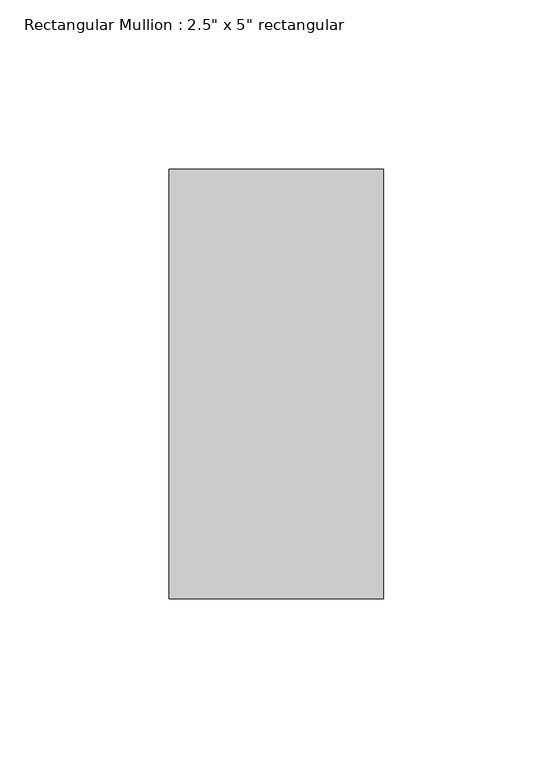
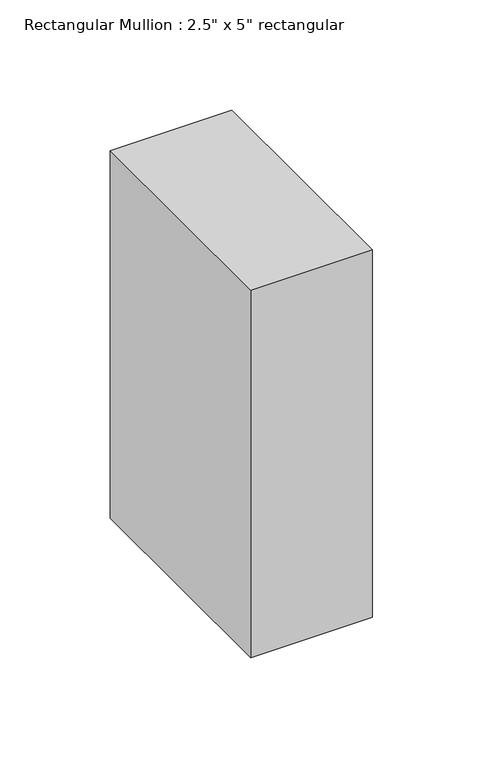
"""IFC4 building model written with IfcOpenShell, lengths in millimetres: member geometry."""

from ifc_helpers import new_model, si_unit, frame, origin, place, context, project, spatial, polyline, outline, extrude, source, transform, mapped, element, save


def member_da94038d(model_context):
    return source(origin(), model_context, "Body", "SweptSolid", [
        extrude(outline(polyline([(31.75, 63.5), (31.75, -63.5), (-31.75, -63.5), (-31.75, 63.5), (31.75, 63.5)])), frame((0.0, 0.0, -203.0665682), z_axis=(0.0, 0.0, 1.0), x_axis=(1.0, 0.0, 0.0)), (0.0, 0.0, 1.0), 203.0665682),
    ])


if __name__ == "__main__":
    model = new_model("IFC4")
    model_context = context("Model", 3, world=origin())
    ifc_project = project(units=[si_unit("LENGTHUNIT", "METRE", prefix="MILLI")], contexts=[model_context])
    site = spatial("IfcSite", under=ifc_project)
    building = spatial("IfcBuilding", under=site)
    placement = place(None, origin())
    member_shape = member_da94038d(model_context)
    element("IfcMember", 1, ObjectType="Rectangular Mullion : 2.5\" x 5\" rectangular", at=placement, inside=building, context=model_context, shape_type="MappedRepresentation", body=[
        mapped(member_shape, transform((0.0, 0.0, 0.0), x_axis=(1.0, 0.0, 0.0), y_axis=(0.0, 1.0, 0.0), z_axis=(0.0, 0.0, 1.0))),
    ])
    save(model, "model.ifc")

# Revit data of these elements
# Type "Rectangular Mullion : 2.5\" x 5\" rectangular"
#   built-in parameter 1007304 = 0.416667 (stored number, unit not read)
#   built-in parameter 1007301 = 0.104167 (stored number, unit not read)
#   built-in parameter 1007300 = 0.104167 (stored number, unit not read)
# Element 1 (IfcMember, "Rectangular Mullion : 2.5\" x 5\" rectangular")
#   Materials on its faces: "Aluminum"
# Materials
#   "Aluminum": class "Metal", colour RGB 247 247 247, transparency 0, Description = "Aluminum 6061", Cost = 0
